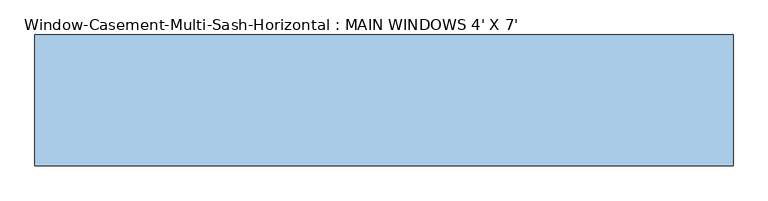
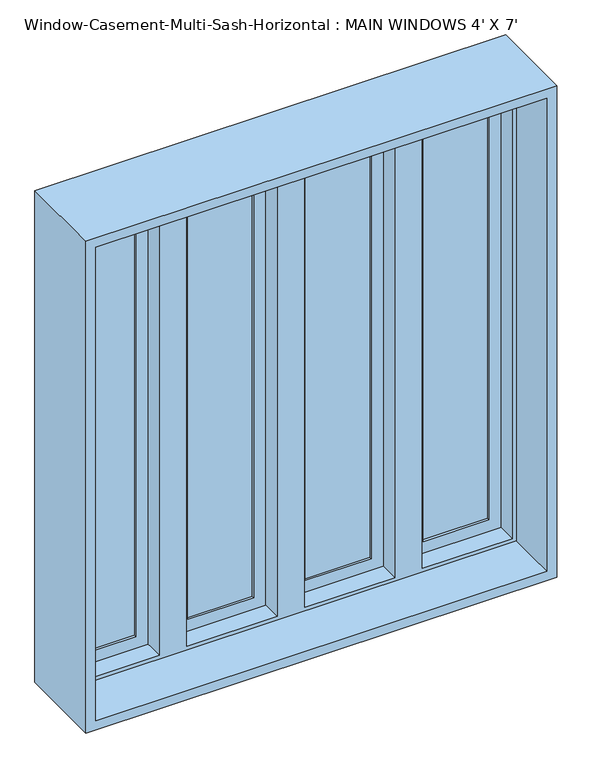
"""IFC4 building model written with IfcOpenShell, lengths in millimetres: window geometry, Window-Casement-Multi-Sash-Horizontal : MAIN WINDOWS 4' X 7'."""

from ifc_helpers import new_model, si_unit, frame, origin, place, context, project, spatial, polyline, outline, extrude, faceted_brep, source, transform, mapped, element, save


def window_casement_multi_sash_horizontal_main_windows_4_x_7_0e27d311(model_context):
    return source(origin(), model_context, "Body", "SolidModel", [
        extrude(outline(polyline([(2235.2, 330.2), (939.8, 330.2), (939.8, 584.2), (2235.2, 584.2), (2235.2, 330.2)]), holes=[polyline([(2193.3296875, 542.3296875), (981.6703125, 542.3296875), (981.6703125, 372.0703125), (2193.3296875, 372.0703125), (2193.3296875, 542.3296875)])]), frame((0.0, 73.025, 0.0), z_axis=(0.0, 1.0, 0.0), x_axis=(0.0, 0.0, 1.0)), (0.0, 0.0, 1.0), 31.75),
        extrude(outline(polyline([(2235.2, -584.2), (939.8, -584.2), (939.8, -330.2), (2235.2, -330.2), (2235.2, -584.2)]), holes=[polyline([(2193.3296875, -372.0703125), (981.6703125, -372.0703125), (981.6703125, -542.3296875), (2193.3296875, -542.3296875), (2193.3296875, -372.0703125)])]), frame((0.0, 73.025, 0.0), z_axis=(0.0, 1.0, 0.0), x_axis=(0.0, 0.0, 1.0)), (0.0, 0.0, 1.0), 31.75),
        extrude(outline(polyline([(-372.0703125, 98.425), (-372.0703125, 92.075), (-542.3296875, 92.075), (-542.3296875, 98.425), (-372.0703125, 98.425)])), frame((0.0, 0.0, 981.6703125), z_axis=(0.0, 0.0, 1.0), x_axis=(1.0, 0.0, 0.0)), (0.0, 0.0, 1.0), 1211.659375),
        extrude(outline(polyline([(-372.0703125, 85.725), (-372.0703125, 79.375), (-542.3296875, 79.375), (-542.3296875, 85.725), (-372.0703125, 85.725)])), frame((0.0, 0.0, 981.6703125), z_axis=(0.0, 0.0, 1.0), x_axis=(1.0, 0.0, 0.0)), (0.0, 0.0, 1.0), 1211.659375),
        extrude(outline(polyline([(542.3296875, 98.425), (542.3296875, 92.075), (372.0703125, 92.075), (372.0703125, 98.425), (542.3296875, 98.425)])), frame((0.0, 0.0, 981.6703125), z_axis=(0.0, 0.0, 1.0), x_axis=(1.0, 0.0, 0.0)), (0.0, 0.0, 1.0), 1211.659375),
        extrude(outline(polyline([(542.3296875, 85.725), (542.3296875, 79.375), (372.0703125, 79.375), (372.0703125, 85.725), (542.3296875, 85.725)])), frame((0.0, 0.0, 981.6703125), z_axis=(0.0, 0.0, 1.0), x_axis=(1.0, 0.0, 0.0)), (0.0, 0.0, 1.0), 1211.659375),
        extrude(outline(polyline([(-67.2703125, 98.425), (-67.2703125, 92.075), (-237.5296875, 92.075), (-237.5296875, 98.425), (-67.2703125, 98.425)])), frame((0.0, 0.0, 981.6703125), z_axis=(0.0, 0.0, 1.0), x_axis=(1.0, 0.0, 0.0)), (0.0, 0.0, 1.0), 1211.659375),
        extrude(outline(polyline([(-67.2703125, 85.725), (-67.2703125, 79.375), (-237.5296875, 79.375), (-237.5296875, 85.725), (-67.2703125, 85.725)])), frame((0.0, 0.0, 981.6703125), z_axis=(0.0, 0.0, 1.0), x_axis=(1.0, 0.0, 0.0)), (0.0, 0.0, 1.0), 1211.659375),
        extrude(outline(polyline([(237.5296875, 98.425), (237.5296875, 92.075), (67.2703125, 92.075), (67.2703125, 98.425), (237.5296875, 98.425)])), frame((0.0, 0.0, 981.6703125), z_axis=(0.0, 0.0, 1.0), x_axis=(1.0, 0.0, 0.0)), (0.0, 0.0, 1.0), 1211.659375),
        extrude(outline(polyline([(237.5296875, 85.725), (237.5296875, 79.375), (67.2703125, 79.375), (67.2703125, 85.725), (237.5296875, 85.725)])), frame((0.0, 0.0, 981.6703125), z_axis=(0.0, 0.0, 1.0), x_axis=(1.0, 0.0, 0.0)), (0.0, 0.0, 1.0), 1211.659375),
        faceted_brep([(-330.2, 73.025, 2235.2), (-584.2, 73.025, 2235.2), (-584.2, 114.3, 2235.2), (584.2, 114.3, 2235.2), (584.2, 73.025, 2235.2), (330.2, 73.025, 2235.2), (330.2, 111.125, 2235.2), (279.4, 111.125, 2235.2), (279.4, 73.025, 2235.2), (25.4, 73.025, 2235.2), (25.4, 111.125, 2235.2), (-25.4, 111.125, 2235.2), (-25.4, 73.025, 2235.2), (-279.4, 73.025, 2235.2), (-279.4, 111.125, 2235.2), (-330.2, 111.125, 2235.2), (-574.0796875, 22.225, 2225.0796875), (-574.0796875, 73.025, 2225.0796875), (-340.3203125, 73.025, 2225.0796875), (-340.3203125, 22.225, 2225.0796875), (574.0796875, 73.025, 2225.0796875), (574.0796875, 22.225, 2225.0796875), (340.3203125, 22.225, 2225.0796875), (340.3203125, 73.025, 2225.0796875), (-269.2796875, 73.025, 2225.0796875), (-35.5203125, 73.025, 2225.0796875), (-35.5203125, 22.225, 2225.0796875), (-269.2796875, 22.225, 2225.0796875), (35.5203125, 73.025, 2225.0796875), (269.2796875, 73.025, 2225.0796875), (269.2796875, 22.225, 2225.0796875), (35.5203125, 22.225, 2225.0796875), (-584.2, -114.3, 2235.2), (-584.2, 22.225, 2235.2), (584.2, 22.225, 2235.2), (584.2, -114.3, 2235.2), (-609.6, 114.3, 2260.6), (-609.6, -114.3, 2260.6), (609.6, -114.3, 2260.6), (609.6, 114.3, 2260.6), (584.2, 114.3, 939.8), (584.2, 73.025, 939.8), (574.0796875, 73.025, 949.9203125), (574.0796875, 22.225, 949.9203125), (584.2, 22.225, 939.8), (584.2, -114.3, 939.8), (609.6, -114.3, 914.4), (609.6, 114.3, 914.4), (330.2, 73.025, 939.8), (-584.2, 114.3, 939.8), (-584.2, 73.025, 939.8), (-330.2, 73.025, 939.8), (-330.2, 111.125, 939.8), (-279.4, 111.125, 939.8), (-279.4, 73.025, 939.8), (-25.4, 73.025, 939.8), (-25.4, 111.125, 939.8), (25.4, 111.125, 939.8), (25.4, 73.025, 939.8), (279.4, 73.025, 939.8), (279.4, 111.125, 939.8), (330.2, 111.125, 939.8), (340.3203125, 73.025, 949.9203125), (340.3203125, 22.225, 949.9203125), (-574.0796875, 73.025, 949.9203125), (-574.0796875, 22.225, 949.9203125), (-340.3203125, 22.225, 949.9203125), (-340.3203125, 73.025, 949.9203125), (-35.5203125, 73.025, 949.9203125), (-269.2796875, 73.025, 949.9203125), (-269.2796875, 22.225, 949.9203125), (-35.5203125, 22.225, 949.9203125), (269.2796875, 73.025, 949.9203125), (35.5203125, 73.025, 949.9203125), (35.5203125, 22.225, 949.9203125), (269.2796875, 22.225, 949.9203125), (-584.2, 22.225, 939.8), (-584.2, -114.3, 939.8), (-609.6, -114.3, 914.4), (-609.6, 114.3, 914.4)], [[[0, 1, 2, 3, 4, 5, 6, 7, 8, 9, 10, 11, 12, 13, 14, 15]], [[16, 17, 18, 19]], [[20, 21, 22, 23]], [[24, 25, 26, 27]], [[28, 29, 30, 31]], [[32, 33, 34, 35]], [[36, 37, 38, 39]], [[4, 3, 40, 41]], [[21, 20, 42, 43]], [[35, 34, 44, 45]], [[39, 38, 46, 47]], [[48, 41, 40, 49, 50, 51, 52, 53, 54, 55, 56, 57, 58, 59, 60, 61]], [[43, 42, 62, 63]], [[64, 65, 66, 67]], [[68, 69, 70, 71]], [[72, 73, 74, 75]], [[45, 44, 76, 77]], [[47, 46, 78, 79]], [[2, 1, 50, 49]], [[4, 41, 48, 5], [20, 23, 62, 42]], [[50, 1, 0, 51], [64, 67, 18, 17]], [[12, 55, 54, 13], [69, 68, 25, 24]], [[8, 59, 58, 9], [73, 72, 29, 28]], [[17, 16, 65, 64]], [[44, 34, 33, 76], [16, 19, 66, 65], [27, 26, 71, 70], [31, 30, 75, 74], [21, 43, 63, 22]], [[33, 32, 77, 76]], [[38, 37, 78, 46], [32, 35, 45, 77]], [[37, 36, 79, 78]], [[36, 39, 47, 79], [3, 2, 49, 40]], [[18, 67, 66, 19]], [[69, 24, 27, 70]], [[53, 14, 13, 54]], [[14, 53, 52, 15]], [[15, 52, 51, 0]], [[25, 68, 71, 26]], [[73, 28, 31, 74]], [[57, 10, 9, 58]], [[10, 57, 56, 11]], [[11, 56, 55, 12]], [[6, 61, 60, 7]], [[7, 60, 59, 8]], [[29, 72, 75, 30]], [[62, 23, 22, 63]], [[61, 6, 5, 48]]]),
        extrude(outline(polyline([(2235.2, 25.4), (939.8, 25.4), (939.8, 279.4), (2235.2, 279.4), (2235.2, 25.4)]), holes=[polyline([(2193.3296875, 237.5296875), (981.6703125, 237.5296875), (981.6703125, 67.2703125), (2193.3296875, 67.2703125), (2193.3296875, 237.5296875)])]), frame((0.0, 73.025, 0.0), z_axis=(0.0, 1.0, 0.0), x_axis=(0.0, 0.0, 1.0)), (0.0, 0.0, 1.0), 31.75),
        extrude(outline(polyline([(2235.2, -279.4), (939.8, -279.4), (939.8, -25.4), (2235.2, -25.4), (2235.2, -279.4)]), holes=[polyline([(2193.3296875, -67.2703125), (981.6703125, -67.2703125), (981.6703125, -237.5296875), (2193.3296875, -237.5296875), (2193.3296875, -67.2703125)])]), frame((0.0, 73.025, 0.0), z_axis=(0.0, 1.0, 0.0), x_axis=(0.0, 0.0, 1.0)), (0.0, 0.0, 1.0), 31.75),
    ])


if __name__ == "__main__":
    model = new_model("IFC4")
    model_context = context("Model", 3, world=origin())
    ifc_project = project(units=[si_unit("LENGTHUNIT", "METRE", prefix="MILLI")], contexts=[model_context])
    site = spatial("IfcSite", under=ifc_project)
    building = spatial("IfcBuilding", under=site)
    placement = place(None, origin())
    window_casement_multi_sash_horizontal_main_windows_4_x_7_shape = window_casement_multi_sash_horizontal_main_windows_4_x_7_0e27d311(model_context)
    element("IfcWindow", 1, ObjectType="Window-Casement-Multi-Sash-Horizontal : MAIN WINDOWS 4' X 7'", at=placement, inside=building, context=model_context, shape_type="MappedRepresentation", body=[
        mapped(window_casement_multi_sash_horizontal_main_windows_4_x_7_shape, transform((0.0, 0.0, 0.0), x_axis=(1.0, 0.0, 0.0), y_axis=(0.0, 1.0, 0.0), z_axis=(0.0, 0.0, 1.0))),
    ])
    save(model, "model.ifc")

# Revit data of these elements
# Type "Window-Casement-Multi-Sash-Horizontal : MAIN WINDOWS 4' X 7'"
#   Type Mark = "21"
#   Fire Rating = "0.5h"
#   Assembly Code = "B2020100"
#   Analytic Construction = "Double glazing - domestic"
#   Window Inset [instance default] = 0' - 0 5/8"
#   Wall Thickness [instance default] = 0' - 6"
#   Visual Light Transmittance = 0.81
#   Thermal Resistance (R) = 1.8146 (h·ft²·°F)/BTU
#   Solar Heat Gain Coefficient = 0.76
#   Rough Width = 4' - 0 1/2"
#   Rough Height = 4' - 5 1/2"
#   Open Window Width = 1' - 0"
#   Heat Transfer Coefficient (U) = 0.5511 BTU/(h·ft²·°F)
#   Height = 4' - 5"
#   Frame Gap 3 [instance default] = 0' - 1 83/128"
#   Frame Gap 2 [instance default] = 0' - 0 5/8"
#   Frame Gap 1 = 0' - 1 51/128"
#   Default Sill Height = 3' - 0"
#   Width = 4' - 0"
#   Frame Material = Metal - Aluminum
#   Glass Panel Material = Glass
#   Wall Closure = (empty or 0)
# Element 1 (IfcWindow, "Window-Casement-Multi-Sash-Horizontal : MAIN WINDOWS 4' X 7'")
#   Wall Thickness = 0' - 9"
#   Materials on its faces: "Metal - Aluminum", "Glass"
# Materials
#   "Metal - Aluminum": class "Metal", colour RGB 247 247 247, transparency 0
#   "Glass": class "Glass", colour RGB 0 128 192, transparency 0.75, Description = "Soda Lime Glass", Cost = 0
